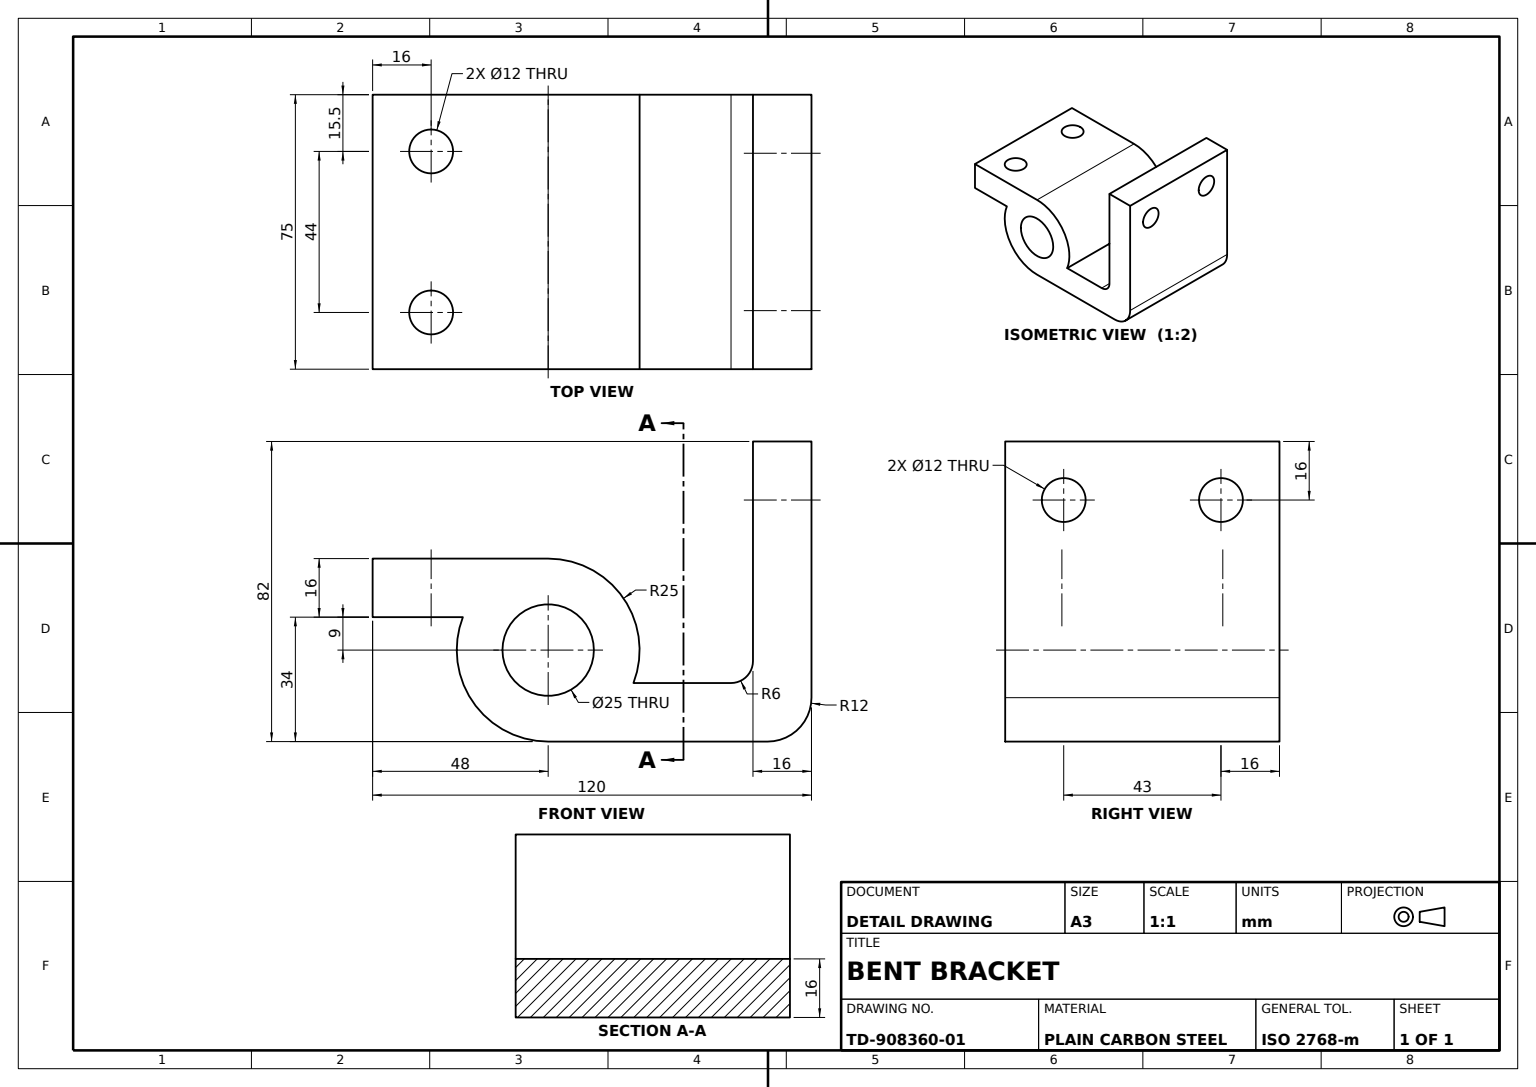
SolidWorks part; units mm, degrees
material "Plain Carbon Steel"
ref_plane "Front Plane" through (0, 0, 0) normal (0, 0, 1) x (1, 0, 0)
ref_plane "Top Plane" through (0, 0, 0) normal (0, 1, 0) x (1, 0, 0)
ref_plane "Right Plane" through (0, 0, 0) normal (1, 0, 0) x (0, 0, -1)
sketch "Bracket Profile Sketch" plane through (0, 0, 0) normal (0, 0, 1) x (1, 0, 0)
  line L0 (0, -25) -> (60, -25)
  line L1 (72, -13) -> (72, 57)
  line L2 (72, 57) -> (56, 57)
  line L3 (56, 57) -> (56, -3)
  line L6 (0, 25) -> (-48, 25)
  line L7 (-48, 25) -> (-48, 9)
  line L8 (-48, 9) -> (-23.3238, 9)
  line L9 (72, -13) -> (72, -9)
  line L10 (50, -9) -> (23.3238, -9)
  arc A0 (-23.3238, 9) -> (0, -25) centre (0, 0) ccw
  arc A1 (23.3238, -9) -> (0, 25) centre (0, 0) ccw
  arc A2 (50, -9) -> (56, -3) centre (50, -3) ccw
  arc A3 (60, -25) -> (72, -13) centre (60, -13) ccw
  dimension "D1" = 50
  dimension "D4" = 6
  dimension "D5" = 12
  dimension "D7" = 25
  dimension "D2" = 120
  dimension "D3" = 56
  dimension "D6" = 16
  dimension "D8" = 24.6762
  dimension "D9" = 26.6762
  dimension "D10" = 82
extrude "Bracket Body" add sketch "Bracket Profile Sketch" along normal blind 75 contours L0 A3 L1 L2 L3 A2 L10 A1 L6 L7 L8 A0
sketch "Flange A Holes Sketch" plane through (0, 25, 0) normal (0, 1, 0) x (1, 0, 0)
  line L0 (0, 0) -> (-48, 0) construction
  line L1 (0, -75) -> (-48, -75) construction
  line L2 (-48, -75) -> (-48, 0) construction
  circle A0 centre (-32, -15.5) radius 6
  circle A1 centre (-32, -59.5) radius 6
  dimension "D1" = 12
  dimension "D2" = 12
  dimension "D8" = 12
  dimension "D3" = 15.5
  dimension "D4" = 15.5
  dimension "D5" = 44
  dimension "D6" = 16
  dimension "D7" = 16
extrude "Flange A Holes 2x" cut sketch "Flange A Holes Sketch" against normal blind 75
sketch "Flange B Holes Sketch" plane through (72, 0, 0) normal (1, 0, 0) x (0, 0, -1)
  line L0 (-75, 57) -> (0, 57) construction
  line L1 (-75, -13) -> (-75, 57) construction
  line L2 (0, -13) -> (0, 57) construction
  circle A0 centre (-59, 41) radius 6
  circle A1 centre (-16, 41) radius 6
  dimension "D1" = 12
  dimension "D2" = 12
  dimension "D7" = 12
  dimension "D3" = 16
  dimension "D4" = 16
  dimension "D5" = 16
  dimension "D6" = 16
extrude "Flange B Holes 2x" cut sketch "Flange B Holes Sketch" against normal blind 75
sketch "Pivot Bore Sketch" plane through (0, 0, 75) normal (0, 0, 1) x (1, 0, 0)
  circle A0 centre (0, 0) radius 12.5
  dimension "D1" = 25
  dimension "D2" = 25
extrude "Pivot Bore" cut sketch "Pivot Bore Sketch" against normal blind 75
